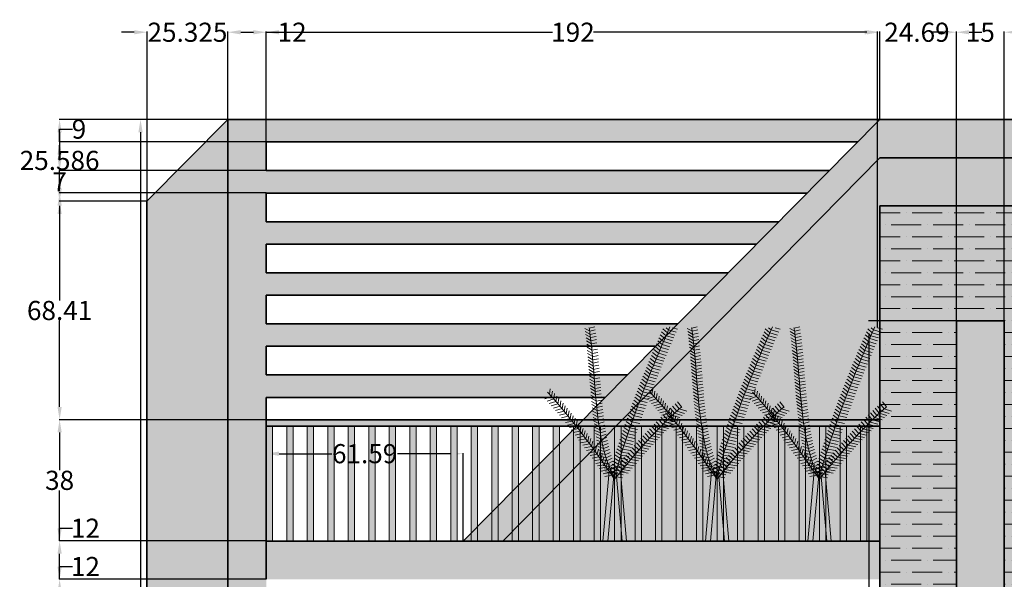
# Model space of a CAD drawing. Units: inches. Extents: x 184 to 649, y 215 to 818.
# Tile 8 of 9: x 184 to 492, y 643 to 818. Entities that reach past the tile are written whole.
import ezdxf

# ---------------------------------------------------------------- set-up
doc = ezdxf.new("R2010")
doc.units = ezdxf.units.IN
doc.header["$MEASUREMENT"] = 0
for name, color, linetype, lineweight in [('A-ANNO-DIMS', 2, 'Continuous', 18), ('A-ELEV', 7, 'Continuous', 35), ('A-ELEV-FILL', 9, 'Continuous', 13), ('A-ELEV-PATT', 8, 'Continuous', 13), ('A-ELEV-RAIL', 8, 'Continuous', 18), ('L-PLNT', 84, 'Continuous', 13)]:
    doc.layers.add(name, color=color, linetype=linetype, lineweight=lineweight)
doc.styles.get("Standard").update_dxf_attribs({"font": 'arial.ttf'})
doc.dimstyles.get("Standard").update_dxf_attribs({"dimtxt": 6, "dimasz": 4, "dimexe": 0.18, "dimexo": 0.0625, "dimgap": 0.09, "dimtad": 0, "dimtih": 1, "dimtoh": 1, "dimdec": 0, "dimzin": 0, "dimdsep": 46, "dimlunit": 3, "dimtxsty": 'Standard', "dimcen": 0.09, "dimadec": 0, "dimazin": 0, "dimtfac": 1, "dimtdec": 0, "dimtofl": 0, "dimtmove": 0, "dimatfit": 3, "dimfxl": 1, "dimtolj": 1, "dimtzin": 0, "dimarcsym": 0})

# ---------------------------------------------------------------- blocks, each defined once
blk = doc.blocks.new('PLANT-PALM')
for p, q in [((274.94, 416.06), (273.31, 416.97)), ((274.8, 417.06), (274.61, 417.16)), ((274.73, 417.05), (276.46, 417.47)), ((274.87, 416.06), (276.6, 416.47)), ((299.15, 415.59), (297.73, 416.77)), ((299.55, 416.5), (298.76, 417.16)), ((299.55, 416.5), (301.94, 415.78)), ((300.78, 417.16), (302.34, 416.68)), ((275.06, 415.07), (273.44, 415.99)), ((275.18, 414.08), (273.57, 415)), ((275.3, 413.08), (273.69, 414.02)), ((275.4, 412.09), (273.8, 413.03)), ((275, 415.07), (276.73, 415.46)), ((275.12, 414.07), (276.85, 414.46)), ((275.23, 413.08), (276.97, 413.45)), ((297.55, 411.92), (296.12, 413.09)), ((297.95, 412.84), (296.52, 414.01)), ((298.34, 413.75), (296.92, 414.93)), ((298.74, 414.67), (297.33, 415.85)), ((298.34, 413.75), (300.74, 413.04)), ((298.74, 414.67), (301.13, 413.96)), ((299.14, 415.59), (301.53, 414.87)), ((275.51, 411.09), (273.9, 412.04)), ((275.6, 410.1), (274, 411.05)), ((275.69, 409.1), (274.1, 410.06)), ((275.34, 412.09), (277.08, 412.45)), ((275.44, 411.09), (277.18, 411.45)), ((275.54, 410.1), (277.28, 410.45)), ((296.38, 409.16), (294.94, 410.32)), ((296.76, 410.08), (295.33, 411.24)), ((297.16, 411), (295.73, 412.16)), ((296.76, 410.08), (299.16, 409.39)), ((297.16, 411), (299.55, 410.3)), ((297.55, 411.92), (299.94, 411.22)), ((297.94, 412.84), (300.34, 412.13)), ((275.78, 408.11), (274.19, 409.06)), ((275.87, 407.11), (274.28, 408.07)), ((275.95, 406.11), (274.36, 407.08)), ((275.63, 409.1), (277.38, 409.45)), ((275.72, 408.1), (277.47, 408.45)), ((275.81, 407.11), (277.55, 407.44)), ((295.22, 406.39), (293.78, 407.54)), ((295.6, 407.31), (294.16, 408.46)), ((295.99, 408.23), (294.55, 409.39)), ((295.6, 407.31), (298.01, 406.64)), ((295.99, 408.24), (298.39, 407.56)), ((296.37, 409.16), (298.78, 408.47)), ((276.03, 405.12), (274.44, 406.08)), ((276.11, 404.12), (274.52, 405.08)), ((276.19, 403.12), (274.6, 404.09)), ((275.89, 406.11), (277.64, 406.45)), ((275.97, 405.11), (277.72, 405.45)), ((276.05, 404.12), (277.8, 404.45)), ((293.71, 402.68), (292.26, 403.82)), ((294.08, 403.61), (292.63, 404.75)), ((294.46, 404.54), (293.01, 405.68)), ((294.84, 405.46), (293.39, 406.61)), ((294.46, 404.54), (296.87, 403.88)), ((294.84, 405.46), (297.25, 404.8)), ((295.22, 406.39), (297.62, 405.72)), ((276.27, 402.13), (274.68, 403.09)), ((276.35, 401.13), (274.75, 402.09)), ((276.43, 400.13), (274.83, 401.09)), ((276.13, 403.12), (277.88, 403.45)), ((276.21, 402.12), (277.96, 402.46)), ((276.29, 401.13), (278.04, 401.46)), ((292.6, 399.9), (291.14, 401.02)), ((292.97, 400.83), (291.51, 401.95)), ((293.34, 401.76), (291.88, 402.89)), ((292.97, 400.83), (295.38, 400.2)), ((293.34, 401.76), (295.75, 401.12)), ((293.71, 402.68), (296.12, 402.04)), ((294.08, 403.61), (296.49, 402.96)), ((262.25, 396.34), (262.49, 398.02)), ((276.51, 399.14), (274.91, 400.09)), ((276.59, 398.14), (274.99, 399.09)), ((276.67, 397.14), (275.07, 398.09)), ((276.37, 400.13), (278.12, 400.47)), ((276.45, 399.13), (278.2, 399.47)), ((276.53, 398.14), (278.28, 398.48)), ((291.51, 397.1), (290.04, 398.21)), ((291.87, 398.03), (290.41, 399.15)), ((292.24, 398.97), (290.77, 400.08)), ((291.87, 398.03), (294.29, 397.42)), ((292.24, 398.97), (294.65, 398.35)), ((292.6, 399.9), (295.02, 399.27)), ((262.93, 395.59), (260.85, 394.94)), ((263.6, 394.85), (261.51, 394.21)), ((262.93, 395.6), (263.18, 397.28)), ((263.6, 394.85), (263.86, 396.53)), ((264.26, 394.11), (264.53, 395.78)), ((264.91, 393.35), (265.2, 395.02)), ((276.76, 396.15), (275.15, 397.08)), ((276.84, 395.15), (275.23, 396.08)), ((276.94, 394.16), (275.32, 395.08)), ((276.62, 397.14), (278.36, 397.49)), ((276.7, 396.14), (278.45, 396.5)), ((276.79, 395.15), (278.54, 395.51)), ((276.89, 394.15), (278.63, 394.52)), ((290.45, 394.3), (288.97, 395.4)), ((290.8, 395.23), (289.33, 396.34)), ((291.16, 396.17), (289.68, 397.27)), ((290.8, 395.23), (293.23, 394.64)), ((291.16, 396.17), (293.58, 395.57)), ((291.51, 397.1), (293.94, 396.5)), ((264.26, 394.1), (262.17, 393.48)), ((264.92, 393.35), (262.82, 392.74)), ((265.57, 392.59), (263.47, 391.99)), ((266.22, 391.82), (264.11, 391.25)), ((265.57, 392.59), (265.86, 394.26)), ((266.21, 391.83), (266.52, 393.5)), ((266.85, 391.06), (267.17, 392.73)), ((267.49, 390.29), (267.81, 391.95)), ((277.03, 393.16), (275.41, 394.07)), ((277.13, 392.17), (275.5, 393.07)), ((277.24, 391.17), (275.6, 392.06)), ((276.99, 393.16), (278.72, 393.54)), ((277.09, 392.16), (278.82, 392.55)), ((277.19, 391.17), (278.93, 391.57)), ((289.07, 390.54), (287.57, 391.62)), ((289.41, 391.48), (287.92, 392.57)), ((289.75, 392.42), (288.27, 393.51)), ((290.1, 393.36), (288.62, 394.45)), ((289.41, 391.48), (291.84, 390.92)), ((289.75, 392.42), (292.18, 391.85)), ((290.1, 393.36), (292.53, 392.78)), ((290.45, 394.3), (292.88, 393.71)), ((301.34, 390.38), (300.06, 391.94)), ((302.08, 391.06), (300.81, 392.62)), ((302.82, 391.73), (301.57, 393.3)), ((303.57, 392.39), (302.33, 393.98)), ((302.82, 391.73), (305.21, 391)), ((266.86, 391.06), (264.75, 390.49)), ((267.49, 390.29), (265.38, 389.73)), ((268.12, 389.51), (266.01, 388.97)), ((268.75, 388.73), (266.64, 388.2)), ((268.12, 389.51), (268.45, 391.17)), ((268.75, 388.73), (269.09, 390.39)), ((269.37, 387.95), (269.72, 389.61)), ((269.99, 387.16), (270.34, 388.82)), ((277.35, 390.18), (275.71, 391.05)), ((277.47, 389.19), (275.82, 390.05)), ((277.6, 388.2), (275.94, 389.04)), ((277.31, 390.18), (279.04, 390.59)), ((277.43, 389.18), (279.15, 389.61)), ((277.56, 388.19), (279.28, 388.63)), ((288.06, 387.72), (286.56, 388.79)), ((288.39, 388.66), (286.89, 389.73)), ((288.73, 389.6), (287.23, 390.68)), ((288.39, 388.66), (290.83, 388.12)), ((288.73, 389.6), (291.16, 389.05)), ((289.07, 390.54), (291.5, 389.98)), ((297.74, 386.91), (296.41, 388.42)), ((298.45, 387.62), (297.13, 389.14)), ((299.16, 388.32), (297.85, 389.85)), ((299.88, 389.01), (298.59, 390.55)), ((299.16, 388.32), (301.58, 387.68)), ((300.61, 389.7), (299.32, 391.25)), ((299.88, 389.01), (302.29, 388.36)), ((300.61, 389.7), (303.01, 389.03)), ((301.34, 390.38), (303.74, 389.69)), ((302.08, 391.06), (304.47, 390.35)), ((269.37, 387.95), (267.26, 387.43)), ((269.99, 387.16), (267.87, 386.65)), ((270.61, 386.37), (268.48, 385.87)), ((271.22, 385.58), (269.09, 385.09)), ((270.6, 386.37), (270.97, 388.03)), ((271.21, 385.58), (271.58, 387.24)), ((271.82, 384.79), (272.2, 386.44)), ((272.42, 383.99), (272.8, 385.64)), ((277.73, 387.21), (276.06, 388.03)), ((277.87, 386.22), (276.2, 387.03)), ((278.02, 385.23), (276.34, 386.02)), ((277.69, 387.2), (279.41, 387.66)), ((277.83, 386.21), (279.55, 386.69)), ((277.99, 385.22), (279.69, 385.72)), ((287.08, 384.88), (285.56, 385.94)), ((287.4, 385.83), (285.89, 386.89)), ((287.73, 386.77), (286.22, 387.84)), ((287.4, 385.83), (289.84, 385.31)), ((287.73, 386.77), (290.17, 386.25)), ((288.06, 387.72), (290.5, 387.18)), ((294.95, 384.05), (293.58, 385.53)), ((295.64, 384.77), (294.28, 386.26)), ((296.33, 385.49), (294.99, 386.98)), ((297.03, 386.2), (295.69, 387.71)), ((296.33, 385.49), (298.76, 384.92)), ((297.03, 386.2), (299.46, 385.61)), ((297.74, 386.91), (300.16, 386.31)), ((298.45, 387.62), (300.87, 387)), ((271.82, 384.79), (269.7, 384.3)), ((272.43, 383.99), (270.3, 383.51)), ((273.03, 383.19), (270.9, 382.72)), ((273.62, 382.39), (271.49, 381.93)), ((273.02, 383.19), (273.41, 384.84)), ((273.62, 382.39), (274.01, 384.04)), ((274.21, 381.58), (274.61, 383.23)), ((274.8, 380.78), (275.21, 382.42)), ((278.18, 384.24), (276.49, 385.01)), ((278.36, 383.26), (276.65, 384)), ((278.54, 382.28), (276.83, 382.99)), ((278.15, 384.24), (279.85, 384.75)), ((278.32, 383.25), (280.02, 383.79)), ((278.51, 382.27), (280.2, 382.83)), ((286.12, 382.04), (284.6, 383.08)), ((286.44, 382.99), (284.92, 384.03)), ((286.76, 383.94), (285.24, 384.98)), ((286.44, 382.99), (288.88, 382.49)), ((286.75, 383.94), (289.2, 383.43)), ((287.08, 384.88), (289.52, 384.37)), ((292.23, 381.11), (290.83, 382.56)), ((292.9, 381.85), (291.51, 383.31)), ((293.58, 382.59), (292.2, 384.05)), ((294.26, 383.32), (292.89, 384.79)), ((293.58, 382.59), (296.02, 382.07)), ((294.26, 383.32), (296.7, 382.79)), ((294.95, 384.05), (297.38, 383.5)), ((295.64, 384.77), (298.07, 384.21)), ((274.22, 381.58), (272.09, 381.13)), ((274.81, 380.78), (272.68, 380.33)), ((275.4, 379.97), (273.26, 379.53)), ((275.99, 379.16), (273.85, 378.72)), ((275.39, 379.97), (275.8, 381.61)), ((275.98, 379.16), (276.39, 380.8)), ((276.56, 378.35), (276.98, 379.99)), ((278.74, 381.3), (277.01, 381.99)), ((277.14, 377.53), (277.56, 379.18)), ((278.95, 380.32), (277.21, 380.98)), ((279.17, 379.35), (277.42, 379.97)), ((278.71, 381.29), (280.39, 381.87)), ((278.92, 380.31), (280.59, 380.92)), ((279.15, 379.34), (280.81, 379.98)), ((284.9, 378.23), (283.36, 379.24)), ((285.2, 379.18), (283.66, 380.2)), ((285.5, 380.14), (283.97, 381.16)), ((285.81, 381.09), (284.28, 382.12)), ((285.2, 379.18), (287.65, 378.72)), ((285.5, 380.14), (287.95, 379.67)), ((285.81, 381.09), (288.26, 380.61)), ((286.12, 382.04), (288.57, 381.55)), ((289.58, 378.12), (288.15, 379.54)), ((290.23, 378.87), (288.81, 380.3)), ((290.9, 379.63), (289.48, 381.06)), ((291.56, 380.37), (290.15, 381.81)), ((290.9, 379.63), (293.35, 379.16)), ((291.56, 380.37), (294.01, 379.89)), ((292.23, 381.11), (294.68, 380.62)), ((292.9, 381.85), (295.35, 381.35)), ((276.57, 378.35), (274.43, 377.92)), ((277.15, 377.53), (275.02, 377.11)), ((277.74, 376.72), (275.6, 376.3)), ((279.41, 378.38), (277.65, 378.97)), ((277.72, 376.72), (278.15, 378.36)), ((279.67, 377.41), (277.9, 377.96)), ((279.95, 376.45), (278.16, 376.96)), ((278.3, 375.9), (278.73, 377.55)), ((278.88, 375.09), (279.31, 376.73)), ((279.39, 378.37), (281.04, 379.04)), ((279.65, 377.4), (281.29, 378.11)), ((279.93, 376.44), (281.55, 377.18)), ((280.23, 375.49), (281.83, 376.27)), ((284.02, 375.36), (282.47, 376.36)), ((284.31, 376.32), (282.76, 377.32)), ((284.6, 377.27), (283.06, 378.28)), ((284.31, 376.32), (286.77, 375.89)), ((284.6, 377.28), (287.06, 376.83)), ((284.9, 378.23), (287.35, 377.78)), ((286.98, 375.08), (285.53, 376.47)), ((287.63, 375.84), (286.18, 377.24)), ((288.27, 376.61), (286.83, 378.01)), ((288.92, 377.36), (287.49, 378.78)), ((288.27, 376.61), (290.73, 376.18)), ((288.92, 377.36), (291.38, 376.93)), ((289.58, 378.12), (292.03, 377.67)), ((290.23, 378.87), (292.69, 378.42)), ((278.31, 375.91), (276.18, 375.49)), ((278.89, 375.09), (276.75, 374.67)), ((279.47, 374.27), (277.33, 373.86)), ((280.05, 373.46), (277.91, 373.04)), ((280.24, 375.49), (278.44, 375.96)), ((280.56, 374.55), (278.75, 374.97)), ((280.9, 373.61), (279.08, 373.97)), ((281.26, 372.67), (279.43, 372.98)), ((279.46, 374.27), (279.88, 375.91)), ((280.03, 373.45), (280.46, 375.09)), ((280.55, 374.54), (282.13, 375.36)), ((280.61, 372.64), (281.04, 374.28)), ((280.89, 373.6), (282.45, 374.46)), ((281.18, 371.82), (281.61, 373.46)), ((281.26, 372.67), (282.79, 373.58)), ((283.18, 372.48), (281.61, 373.46)), ((283.45, 373.44), (281.89, 374.43)), ((283.73, 374.4), (282.18, 375.39)), ((284.44, 371.99), (282.97, 373.36)), ((283.45, 373.44), (285.92, 373.04)), ((285.07, 372.76), (283.61, 374.14)), ((283.73, 374.4), (286.2, 373.99)), ((284.02, 375.36), (286.48, 374.94)), ((285.71, 373.54), (284.24, 374.92)), ((286.34, 374.31), (284.89, 375.7)), ((285.71, 373.54), (288.17, 373.15)), ((286.34, 374.31), (288.81, 373.91)), ((286.98, 375.08), (289.45, 374.67)), ((287.63, 375.84), (290.09, 375.43)), ((280.62, 372.64), (278.48, 372.23)), ((281.2, 371.82), (279.05, 371.41)), ((281.77, 371), (279.63, 370.59)), ((281.65, 371.75), (279.81, 372)), ((282.9, 371.52), (281.33, 372.49)), ((281.65, 371.75), (283.15, 372.7)), ((281.77, 371), (282.24, 372.12)), ((282.07, 370.84), (283.54, 371.85)), ((282.63, 370.56), (285.1, 370.19)), ((282.9, 371.52), (285.37, 371.14)), ((283.18, 372.48), (285.64, 372.09)), ((284.44, 371.99), (286.91, 371.62)), ((285.07, 372.76), (287.54, 372.39))]:
    blk.add_line(p, q)
blk.add_open_spline([(274.68, 417.16), (274.77, 416.57), (276.95, 400.47), (276.36, 381.5), (282.64, 369.73)], degree=3, knots=[87.299959, 87.299959, 87.299959, 87.299959, 88.780677, 127.704389, 127.704389, 127.704389, 127.704389])
for points in [[(282.63, 370.56), (286.61, 384.99), (292.84, 401.43), (299.95, 417.41)], [(282.55, 369.88), (275.93, 379.33), (269.31, 388.78), (261.65, 396.98)], [(282.64, 369.73), (290.67, 379.89), (297.61, 387.15), (303.65, 392.43)]]:
    blk.add_open_spline(points, degree=3)
blk = doc.blocks.new('PLANT-STEM')
for p, q in [((319.07, 530.29), (317.11, 508.48)), ((320.61, 530.15), (318.67, 508.48)), ((322.56, 530.1), (324.44, 508.48)), ((320.76, 528.67), (320.77, 508.48)), ((321.21, 529.98), (323.08, 508.48))]:
    blk.add_line(p, q)
blk = doc.blocks.new('*D10')
at = {"layer": 'A-ANNO-DIMS', "color": 0, "lineweight": -2, "transparency": 16777216}
for p, q in [((248.91, 786.73), (221.44, 786.73)), ((221.62, 782.73), (221.62, 519.88)), ((221.62, 250.73), (221.62, 513.57)), ((248.91, 246.73), (221.44, 246.73))]:
    blk.add_line(p, q, dxfattribs=at)
at = {"layer": 'A-ANNO-DIMS', "color": 0, "transparency": 16777216}
for points in [[(220.96, 782.73), (222.29, 782.73), (221.62, 786.73)], [(220.96, 250.73), (222.29, 250.73), (221.62, 246.73)]]:
    blk.add_solid(points, dxfattribs=at)
at = {"layer": 'Defpoints', "color": 0, "transparency": 16777216}
for p in [(221.62, 786.73), (248.97, 786.73), (248.97, 246.73)]:
    blk.add_point(p, dxfattribs=at)
at = {"layer": 'A-ANNO-DIMS', "color": 0, "transparency": 16777216, "insert": (221.62, 516.73), "char_height": 6, "attachment_point": 5}
blk.add_mtext('\\A1;540', dxfattribs=at)
blk = doc.blocks.new('*D19')
at = {"layer": 'A-ANNO-DIMS', "color": 0, "lineweight": -2, "transparency": 16777216}
for p, q in [((219.65, 814.08), (215.65, 814.08)), ((223.65, 761.2), (223.65, 814.26)), ((248.97, 786.79), (248.97, 814.26)), ((252.97, 814.08), (256.97, 814.08))]:
    blk.add_line(p, q, dxfattribs=at)
at = {"layer": 'A-ANNO-DIMS', "color": 0, "transparency": 16777216}
for points in [[(219.65, 814.74), (219.65, 813.41), (223.65, 814.08)], [(252.97, 814.74), (252.97, 813.41), (248.97, 814.08)]]:
    blk.add_solid(points, dxfattribs=at)
at = {"layer": 'Defpoints', "color": 0, "transparency": 16777216}
for p in [(248.97, 814.08), (248.97, 786.73), (223.65, 761.14)]:
    blk.add_point(p, dxfattribs=at)
at = {"layer": 'A-ANNO-DIMS', "color": 0, "transparency": 16777216, "insert": (236.31, 814.08), "char_height": 6, "attachment_point": 5}
blk.add_mtext('\\A1;25.325', dxfattribs=at)
blk = doc.blocks.new('*D20')
at = {"layer": 'A-ANNO-DIMS', "color": 0, "lineweight": -2, "transparency": 16777216}
for p, q in [((248.97, 786.79), (248.97, 814.26)), ((252.97, 814.08), (256.97, 814.08)), ((260.97, 779.79), (260.97, 814.26)), ((260.97, 814.08), (264.97, 814.08))]:
    blk.add_line(p, q, dxfattribs=at)
at = {"layer": 'A-ANNO-DIMS', "color": 0, "transparency": 16777216}
for points in [[(252.97, 814.74), (252.97, 813.41), (248.97, 814.08)], [(256.97, 814.74), (256.97, 813.41), (260.97, 814.08)]]:
    blk.add_solid(points, dxfattribs=at)
at = {"layer": 'Defpoints', "color": 0, "transparency": 16777216}
for p in [(260.97, 814.08), (248.97, 786.73), (260.97, 779.73)]:
    blk.add_point(p, dxfattribs=at)
at = {"layer": 'A-ANNO-DIMS', "color": 0, "transparency": 16777216, "insert": (269.05, 814.08), "char_height": 6, "attachment_point": 5}
blk.add_mtext('\\A1;12', dxfattribs=at)
blk = doc.blocks.new('*D21')
at = {"layer": 'A-ANNO-DIMS', "color": 0, "lineweight": -2, "transparency": 16777216}
for p, q in [((260.97, 779.79), (260.97, 814.26)), ((264.97, 814.08), (350.57, 814.08)), ((448.97, 814.08), (363.38, 814.08)), ((452.97, 786.79), (452.97, 814.26))]:
    blk.add_line(p, q, dxfattribs=at)
at = {"layer": 'A-ANNO-DIMS', "color": 0, "transparency": 16777216}
for points in [[(264.97, 814.74), (264.97, 813.41), (260.97, 814.08)], [(448.97, 814.74), (448.97, 813.41), (452.97, 814.08)]]:
    blk.add_solid(points, dxfattribs=at)
at = {"layer": 'Defpoints', "color": 0, "transparency": 16777216}
for p in [(452.97, 814.08), (452.97, 786.73), (260.97, 779.73)]:
    blk.add_point(p, dxfattribs=at)
at = {"layer": 'A-ANNO-DIMS', "color": 0, "transparency": 16777216, "insert": (356.97, 814.08), "char_height": 6, "attachment_point": 5}
blk.add_mtext('\\A1;192', dxfattribs=at)
blk = doc.blocks.new('*D22')
at = {"layer": 'A-ANNO-DIMS', "color": 0, "lineweight": -2, "transparency": 16777216}
for p, q in [((448.28, 814.08), (444.28, 814.08)), ((452.28, 721.59), (452.28, 814.26)), ((476.97, 723.79), (476.97, 814.26)), ((480.97, 814.08), (484.97, 814.08))]:
    blk.add_line(p, q, dxfattribs=at)
at = {"layer": 'A-ANNO-DIMS', "color": 0, "transparency": 16777216}
for points in [[(448.28, 814.74), (448.28, 813.41), (452.28, 814.08)], [(480.97, 814.74), (480.97, 813.41), (476.97, 814.08)]]:
    blk.add_solid(points, dxfattribs=at)
at = {"layer": 'Defpoints', "color": 0, "transparency": 16777216}
for p in [(476.97, 814.08), (452.28, 721.53), (476.97, 723.73)]:
    blk.add_point(p, dxfattribs=at)
at = {"layer": 'A-ANNO-DIMS', "color": 0, "transparency": 16777216, "insert": (464.63, 814.08), "char_height": 6, "attachment_point": 5}
blk.add_mtext('\\A1;24.69', dxfattribs=at)
blk = doc.blocks.new('*D23')
at = {"layer": 'A-ANNO-DIMS', "color": 0, "lineweight": -2, "transparency": 16777216}
for p, q in [((472.97, 814.08), (468.97, 814.08)), ((476.97, 723.79), (476.97, 814.26)), ((491.97, 723.79), (491.97, 814.26)), ((495.97, 814.08), (499.97, 814.08))]:
    blk.add_line(p, q, dxfattribs=at)
at = {"layer": 'A-ANNO-DIMS', "color": 0, "transparency": 16777216}
for points in [[(472.97, 814.74), (472.97, 813.41), (476.97, 814.08)], [(495.97, 814.74), (495.97, 813.41), (491.97, 814.08)]]:
    blk.add_solid(points, dxfattribs=at)
at = {"layer": 'Defpoints', "color": 0, "transparency": 16777216}
for p in [(491.97, 814.08), (476.97, 723.73), (491.97, 723.73)]:
    blk.add_point(p, dxfattribs=at)
at = {"layer": 'A-ANNO-DIMS', "color": 0, "transparency": 16777216, "insert": (484.47, 814.08), "char_height": 6, "attachment_point": 5}
blk.add_mtext('\\A1;15', dxfattribs=at)
blk = doc.blocks.new('*D39')
at = {"layer": 'A-ANNO-DIMS', "color": 0, "lineweight": -2, "transparency": 16777216}
for p, q in [((196.3, 642.73), (196.3, 646.73)), ((196.3, 646.73), (200.3, 646.73)), ((260.91, 642.73), (196.12, 642.73)), ((196.3, 634.73), (196.3, 638.73)), ((260.91, 630.73), (196.12, 630.73))]:
    blk.add_line(p, q, dxfattribs=at)
at = {"layer": 'A-ANNO-DIMS', "color": 0, "transparency": 16777216}
for points in [[(195.63, 638.73), (196.96, 638.73), (196.3, 642.73)], [(195.63, 634.73), (196.96, 634.73), (196.3, 630.73)]]:
    blk.add_solid(points, dxfattribs=at)
at = {"layer": 'Defpoints', "color": 0, "transparency": 16777216}
for p in [(196.3, 642.73), (260.97, 642.73), (260.97, 630.73)]:
    blk.add_point(p, dxfattribs=at)
at = {"layer": 'A-ANNO-DIMS', "color": 0, "transparency": 16777216, "insert": (204.37, 646.73), "char_height": 6, "attachment_point": 5}
blk.add_mtext('\\A1;12', dxfattribs=at)
blk = doc.blocks.new('*D40')
at = {"layer": 'A-ANNO-DIMS', "color": 0, "lineweight": -2, "transparency": 16777216}
for p, q in [((196.3, 654.73), (196.3, 658.73)), ((196.3, 658.73), (200.3, 658.73)), ((260.91, 654.73), (196.12, 654.73)), ((196.3, 646.73), (196.3, 650.73)), ((260.91, 642.73), (196.12, 642.73))]:
    blk.add_line(p, q, dxfattribs=at)
at = {"layer": 'A-ANNO-DIMS', "color": 0, "transparency": 16777216}
for points in [[(195.63, 650.73), (196.96, 650.73), (196.3, 654.73)], [(195.63, 646.73), (196.96, 646.73), (196.3, 642.73)]]:
    blk.add_solid(points, dxfattribs=at)
at = {"layer": 'Defpoints', "color": 0, "transparency": 16777216}
for p in [(196.3, 654.73), (260.97, 654.73), (260.97, 642.73)]:
    blk.add_point(p, dxfattribs=at)
at = {"layer": 'A-ANNO-DIMS', "color": 0, "transparency": 16777216, "insert": (204.37, 658.73), "char_height": 6, "attachment_point": 5}
blk.add_mtext('\\A1;12', dxfattribs=at)
blk = doc.blocks.new('*D41')
at = {"layer": 'A-ANNO-DIMS', "color": 0, "lineweight": -2, "transparency": 16777216}
for p, q in [((260.91, 692.73), (196.12, 692.73)), ((196.3, 688.73), (196.3, 676.88)), ((196.3, 658.73), (196.3, 670.57)), ((260.91, 654.73), (196.12, 654.73))]:
    blk.add_line(p, q, dxfattribs=at)
at = {"layer": 'A-ANNO-DIMS', "color": 0, "transparency": 16777216}
for points in [[(195.63, 688.73), (196.96, 688.73), (196.3, 692.73)], [(195.63, 658.73), (196.96, 658.73), (196.3, 654.73)]]:
    blk.add_solid(points, dxfattribs=at)
at = {"layer": 'Defpoints', "color": 0, "transparency": 16777216}
for p in [(196.3, 692.73), (260.97, 692.73), (260.97, 654.73)]:
    blk.add_point(p, dxfattribs=at)
at = {"layer": 'A-ANNO-DIMS', "color": 0, "transparency": 16777216, "insert": (196.3, 673.73), "char_height": 6, "attachment_point": 5}
blk.add_mtext('\\A1;38', dxfattribs=at)
blk = doc.blocks.new('*D42')
at = {"layer": 'A-ANNO-DIMS', "color": 0, "lineweight": -2, "transparency": 16777216}
for p, q in [((223.58, 761.14), (196.12, 761.14)), ((196.3, 757.14), (196.3, 730.09)), ((196.3, 696.73), (196.3, 723.78)), ((260.91, 692.73), (196.12, 692.73))]:
    blk.add_line(p, q, dxfattribs=at)
at = {"layer": 'A-ANNO-DIMS', "color": 0, "transparency": 16777216}
for points in [[(195.63, 757.14), (196.96, 757.14), (196.3, 761.14)], [(195.63, 696.73), (196.96, 696.73), (196.3, 692.73)]]:
    blk.add_solid(points, dxfattribs=at)
at = {"layer": 'Defpoints', "color": 0, "transparency": 16777216}
for p in [(196.3, 761.14), (223.65, 761.14), (260.97, 692.73)]:
    blk.add_point(p, dxfattribs=at)
at = {"layer": 'A-ANNO-DIMS', "color": 0, "transparency": 16777216, "insert": (196.3, 726.93), "char_height": 6, "attachment_point": 5}
blk.add_mtext('\\A1;68.41', dxfattribs=at)
blk = doc.blocks.new('*D43')
at = {"layer": 'A-ANNO-DIMS', "color": 0, "lineweight": -2, "transparency": 16777216}
for p, q in [((248.91, 786.73), (196.12, 786.73)), ((196.3, 782.73), (196.3, 777.09)), ((196.3, 765.14), (196.3, 770.78)), ((223.58, 761.14), (196.12, 761.14))]:
    blk.add_line(p, q, dxfattribs=at)
at = {"layer": 'A-ANNO-DIMS', "color": 0, "transparency": 16777216}
for points in [[(195.63, 782.73), (196.96, 782.73), (196.3, 786.73)], [(195.63, 765.14), (196.96, 765.14), (196.3, 761.14)]]:
    blk.add_solid(points, dxfattribs=at)
at = {"layer": 'Defpoints', "color": 0, "transparency": 16777216}
for p in [(196.3, 786.73), (248.97, 786.73), (223.65, 761.14)]:
    blk.add_point(p, dxfattribs=at)
at = {"layer": 'A-ANNO-DIMS', "color": 0, "transparency": 16777216, "insert": (196.3, 773.93), "char_height": 6, "attachment_point": 5}
blk.add_mtext('\\A1;25.586', dxfattribs=at)
blk = doc.blocks.new('*D54')
at = {"layer": 'A-ANNO-DIMS', "color": 0, "lineweight": -2, "transparency": 16777216}
for p, q in [((196.3, 779.73), (196.3, 783.73)), ((196.3, 783.73), (200.3, 783.73)), ((260.91, 779.73), (196.12, 779.73)), ((196.3, 774.73), (196.3, 775.73)), ((260.91, 770.73), (196.12, 770.73))]:
    blk.add_line(p, q, dxfattribs=at)
at = {"layer": 'A-ANNO-DIMS', "color": 0, "transparency": 16777216}
for points in [[(195.63, 775.73), (196.96, 775.73), (196.3, 779.73)], [(195.63, 774.73), (196.96, 774.73), (196.3, 770.73)]]:
    blk.add_solid(points, dxfattribs=at)
at = {"layer": 'Defpoints', "color": 0, "transparency": 16777216}
for p in [(196.3, 779.73), (260.97, 779.73), (260.97, 770.73)]:
    blk.add_point(p, dxfattribs=at)
at = {"layer": 'A-ANNO-DIMS', "color": 0, "transparency": 16777216, "insert": (202.36, 783.73), "char_height": 6, "attachment_point": 5}
blk.add_mtext('\\A1;9', dxfattribs=at)
blk = doc.blocks.new('*D55')
at = {"layer": 'A-ANNO-DIMS', "color": 0, "lineweight": -2, "transparency": 16777216}
for p, q in [((196.3, 774.73), (196.3, 778.73)), ((260.91, 770.73), (196.12, 770.73)), ((260.91, 763.73), (196.12, 763.73)), ((196.3, 759.73), (196.3, 755.73))]:
    blk.add_line(p, q, dxfattribs=at)
at = {"layer": 'A-ANNO-DIMS', "color": 0, "transparency": 16777216}
for points in [[(195.63, 774.73), (196.96, 774.73), (196.3, 770.73)], [(195.63, 759.73), (196.96, 759.73), (196.3, 763.73)]]:
    blk.add_solid(points, dxfattribs=at)
at = {"layer": 'Defpoints', "color": 0, "transparency": 16777216}
for p in [(196.3, 770.73), (260.97, 770.73), (260.97, 763.73)]:
    blk.add_point(p, dxfattribs=at)
at = {"layer": 'A-ANNO-DIMS', "color": 0, "transparency": 16777216, "insert": (196.3, 767.23), "char_height": 6, "attachment_point": 5}
blk.add_mtext('\\A1;7', dxfattribs=at)
blk = doc.blocks.new('*D56')
at = {"layer": 'A-ANNO-DIMS', "color": 0, "lineweight": -2, "transparency": 16777216}
for p, q in [((260.97, 654.79), (260.97, 682.26)), ((264.97, 682.08), (281.53, 682.08)), ((318.57, 682.08), (302.01, 682.08)), ((322.57, 654.79), (322.57, 682.26))]:
    blk.add_line(p, q, dxfattribs=at)
at = {"layer": 'A-ANNO-DIMS', "color": 0, "transparency": 16777216}
for points in [[(264.97, 682.74), (264.97, 681.41), (260.97, 682.08)], [(318.57, 682.74), (318.57, 681.41), (322.57, 682.08)]]:
    blk.add_solid(points, dxfattribs=at)
at = {"layer": 'Defpoints', "color": 0, "transparency": 16777216}
for p in [(322.57, 682.08), (260.97, 654.73), (322.57, 654.73)]:
    blk.add_point(p, dxfattribs=at)
at = {"layer": 'A-ANNO-DIMS', "color": 0, "transparency": 16777216, "insert": (291.77, 682.08), "char_height": 6, "attachment_point": 5}
blk.add_mtext('\\A1;61.59', dxfattribs=at)
blk = doc.blocks.new('*D63')
at = {"layer": 'A-ANNO-DIMS', "color": 0, "lineweight": -2, "transparency": 16777216}
for p, q in [((476.91, 723.73), (449.44, 723.73)), ((449.62, 719.73), (449.62, 603.63)), ((449.62, 481.22), (449.62, 597.32)), ((476.91, 477.22), (449.44, 477.22))]:
    blk.add_line(p, q, dxfattribs=at)
at = {"layer": 'A-ANNO-DIMS', "color": 0, "transparency": 16777216}
for points in [[(448.96, 719.73), (450.29, 719.73), (449.62, 723.73)], [(448.96, 481.22), (450.29, 481.22), (449.62, 477.22)]]:
    blk.add_solid(points, dxfattribs=at)
at = {"layer": 'Defpoints', "color": 0, "transparency": 16777216}
for p in [(449.62, 723.73), (476.97, 723.73), (476.97, 477.22)]:
    blk.add_point(p, dxfattribs=at)
at = {"layer": 'A-ANNO-DIMS', "color": 0, "transparency": 16777216, "insert": (449.62, 600.47), "char_height": 6, "attachment_point": 5}
blk.add_mtext('\\A1;246.5', dxfattribs=at)

msp = doc.modelspace()

# ---------------------------------------------------------------- hatches: boundary and pattern name
at = {"layer": 'A-ELEV-FILL'}
h = msp.add_hatch(color=256, dxfattribs=at)
h.dxf.hatch_style = 1
h.paths.add_polyline_path([(248.9726, 786.7265), (223.6471, 761.141), (223.6471, 257.141), (248.9726, 246.7265)])
h = msp.add_hatch(color=256, dxfattribs=at)
h.dxf.hatch_style = 1
h.paths.add_polyline_path([(452.9726, 369.7265), (248.9726, 369.7265), (248.9726, 246.7265), (275.9726, 246.7265), (275.9726, 328.7265), (437.9726, 328.7265), (437.9726, 246.7265), (446.6666, 246.7265), (452.9726, 282.7265)])
h.paths.add_polyline_path([(275.9726, 340.7265), (275.9726, 354.7265), (437.9726, 354.7265), (437.9726, 340.7265)], flags=16)
h.paths.add_polyline_path([(452.9726, 510.7265), (260.9726, 510.7265), (260.9726, 642.7265), (260.9726, 699.7265), (367.0226, 699.7265), (373.9381, 706.7265), (260.9726, 706.7265), (260.9726, 715.7265), (382.8295, 715.7265), (389.745, 722.7265), (260.9726, 722.7265), (260.9726, 731.7265), (398.6364, 731.7265), (405.5519, 738.7265), (260.9726, 738.7265), (260.9726, 747.7265), (414.4433, 747.7265), (421.3588, 754.7265), (260.9726, 754.7265), (260.9726, 763.7265), (430.2502, 763.7265), (437.1657, 770.7265), (260.9726, 770.7265), (260.9726, 779.7265), (446.057, 779.7265), (452.9726, 786.7265), (248.9726, 786.7265), (248.9726, 369.7265), (260.9726, 369.7265), (260.9726, 498.7265), (452.9726, 498.7265)])
h = msp.add_hatch(color=256, dxfattribs=at)
h.dxf.hatch_style = 1
h.paths.add_polyline_path([(608.9726, 786.7265), (452.9726, 786.7265), (360.1071, 692.7265), (372.3627, 692.7265), (452.9726, 774.7265), (596.9726, 774.7265), (596.9726, 369.7265), (581.9726, 369.7265), (581.9726, 282.7265), (594.8393, 246.7265), (608.9726, 246.7265)])
h = msp.add_hatch(color=256, dxfattribs=at)
h.dxf.hatch_style = 1
h.paths.add_polyline_path([(596.9726, 774.7265), (452.9726, 774.7265), (372.3627, 692.7265), (386.4196, 692.7265), (452.9726, 759.7265), (581.9726, 759.7265)])
h = msp.add_hatch(color=256, dxfattribs=at)
h.dxf.hatch_style = 1
h.paths.add_polyline_path([(452.9726, 759.7265), (386.4196, 692.7265), (452.9726, 692.7265)])
h = msp.add_hatch(color=256, dxfattribs=at)
h.dxf.hatch_style = 1
h.paths.add_polyline_path([(521.9726, 759.7265), (452.9726, 759.7265), (452.9726, 441.2233), (521.9726, 441.2233)])
h.paths.add_polyline_path([(491.9726, 477.2233), (476.9726, 477.2233), (476.9726, 723.7265), (491.9726, 723.7265)], flags=16)
h = msp.add_hatch(color=256, dxfattribs=at)
h.dxf.hatch_style = 1
h.paths.add_polyline_path([(491.9726, 723.7265), (476.9726, 723.7265), (476.9726, 477.2233), (491.9726, 477.2233)])
h = msp.add_hatch(color=256, dxfattribs=at)
h.dxf.hatch_style = 1
h.paths.add_polyline_path([(360.1071, 692.7265), (260.9726, 692.7265), (260.9726, 690.7265), (358.1312, 690.7265)])
h.paths.add_polyline_path([(262.9726, 690.7265), (260.9726, 690.7265), (260.9726, 654.7265), (262.9726, 654.7265)])
h.paths.add_polyline_path([(269.3864, 690.7265), (267.3864, 690.7265), (267.3864, 654.7265), (269.3864, 654.7265)])
h.paths.add_polyline_path([(275.8001, 690.7265), (273.8001, 690.7265), (273.8001, 654.7265), (275.8001, 654.7265)])
h.paths.add_polyline_path([(282.2139, 690.7265), (280.2139, 690.7265), (280.2139, 654.7265), (282.2139, 654.7265)])
h.paths.add_polyline_path([(288.6277, 690.7265), (286.6277, 690.7265), (286.6277, 654.7265), (288.6277, 654.7265)])
h.paths.add_polyline_path([(295.0415, 690.7265), (293.0415, 690.7265), (293.0415, 654.7265), (295.0415, 654.7265)])
h.paths.add_polyline_path([(301.4553, 690.7265), (299.4553, 690.7265), (299.4553, 654.7265), (301.4553, 654.7265)])
h.paths.add_polyline_path([(307.8691, 690.7265), (305.8691, 690.7265), (305.8691, 654.7265), (307.8691, 654.7265)])
h.paths.add_polyline_path([(314.2829, 690.7265), (312.2829, 690.7265), (312.2829, 654.7265), (314.2829, 654.7265)])
h.paths.add_polyline_path([(320.6967, 690.7265), (318.6967, 690.7265), (318.6967, 654.7265), (320.6967, 654.7265)])
h.paths.add_polyline_path([(327.1105, 690.7265), (325.1105, 690.7265), (325.1105, 657.3024), (327.1105, 659.3269)])
h.paths.add_polyline_path([(333.5243, 690.7265), (331.5243, 690.7265), (331.5243, 663.7946), (333.5243, 665.819)])
h.paths.add_polyline_path([(339.9381, 690.7265), (337.9381, 690.7265), (337.9381, 670.2867), (339.9381, 672.3112)])
h.paths.add_polyline_path([(346.3519, 690.7265), (344.3519, 690.7265), (344.3519, 676.7789), (346.3519, 678.8033)])
h.paths.add_polyline_path([(352.7657, 690.7265), (350.7657, 690.7265), (350.7657, 683.271), (352.7657, 685.2955)])
h.paths.add_polyline_path([(358.1312, 690.7265), (357.1795, 690.7265), (357.1795, 689.7632)], flags=17)
h.paths.add_polyline_path([(372.3627, 692.7265), (360.1071, 692.7265), (358.1312, 690.7265), (370.3966, 690.7265)])
h.paths.add_polyline_path([(452.9726, 692.7265), (372.3627, 692.7265), (370.3966, 690.7265), (452.9726, 690.7265)])
h.paths.add_polyline_path([(448.9726, 690.7265), (446.9726, 690.7265), (446.9726, 654.7265), (448.9726, 654.7265)])
h.paths.add_polyline_path([(442.5588, 690.7265), (440.5588, 690.7265), (440.5588, 654.7265), (442.5588, 654.7265)])
h.paths.add_polyline_path([(436.145, 690.7265), (434.145, 690.7265), (434.145, 654.7265), (436.145, 654.7265)])
h.paths.add_polyline_path([(429.7312, 690.7265), (427.7312, 690.7265), (427.7312, 654.7265), (429.7312, 654.7265)])
h.paths.add_polyline_path([(423.3174, 690.7265), (421.3174, 690.7265), (421.3174, 654.7265), (423.3174, 654.7265)])
h.paths.add_polyline_path([(416.9036, 690.7265), (414.9036, 690.7265), (414.9036, 654.7265), (416.9036, 654.7265)])
h.paths.add_polyline_path([(410.4898, 690.7265), (408.4898, 690.7265), (408.4898, 654.7265), (410.4898, 654.7265)])
h.paths.add_polyline_path([(404.076, 690.7265), (402.076, 690.7265), (402.076, 654.7265), (404.076, 654.7265)])
h.paths.add_polyline_path([(397.6622, 690.7265), (395.6622, 690.7265), (395.6622, 654.7265), (397.6622, 654.7265)])
h.paths.add_polyline_path([(391.2484, 690.7265), (389.2484, 690.7265), (389.2484, 654.7265), (391.2484, 654.7265)])
h.paths.add_polyline_path([(384.8346, 690.7265), (382.8346, 690.7265), (382.8346, 654.7265), (384.8346, 654.7265)])
h.paths.add_polyline_path([(378.4208, 690.7265), (376.4208, 690.7265), (376.4208, 654.7265), (378.4208, 654.7265)])
h.paths.add_polyline_path([(372.007, 690.7265), (370.3966, 690.7265), (370.007, 690.3302), (370.007, 654.7265), (372.007, 654.7265)])
h.paths.add_polyline_path([(365.5932, 685.8403), (363.5932, 683.8058), (363.5932, 654.7265), (365.5932, 654.7265)])
h.paths.add_polyline_path([(359.1795, 679.3159), (357.1795, 677.2814), (357.1795, 654.7265), (359.1795, 654.7265)])
h.paths.add_polyline_path([(352.7657, 672.7915), (350.7657, 670.757), (350.7657, 654.7265), (352.7657, 654.7265)])
h.paths.add_polyline_path([(346.3519, 666.2671), (344.3519, 664.2326), (344.3519, 654.7265), (346.3519, 654.7265)])
h.paths.add_polyline_path([(339.9381, 659.7427), (337.9381, 657.7082), (337.9381, 654.7265), (339.9381, 654.7265)])
h.paths.add_polyline_path([(327.1105, 659.3269), (325.1105, 657.3024), (325.1105, 654.7265), (327.1105, 654.7265)])
h.paths.add_polyline_path([(333.5243, 665.819), (331.5243, 663.7946), (331.5243, 654.7265), (333.5243, 654.7265)])
h.paths.add_polyline_path([(339.9381, 672.3112), (337.9381, 670.2867), (337.9381, 657.7082), (339.9381, 659.7427)])
h.paths.add_polyline_path([(346.3519, 678.8033), (344.3519, 676.7789), (344.3519, 664.2326), (346.3519, 666.2671)])
h.paths.add_polyline_path([(352.7657, 685.2955), (350.7657, 683.271), (350.7657, 670.757), (352.7657, 672.7915)])
h.paths.add_polyline_path([(359.1795, 690.7265), (358.1312, 690.7265), (357.1795, 689.7632), (357.1795, 677.2814), (359.1795, 679.3159)])
h.paths.add_polyline_path([(365.5932, 690.7265), (363.5932, 690.7265), (363.5932, 683.8058), (365.5932, 685.8403)])
h.paths.add_polyline_path([(370.3966, 690.7265), (370.007, 690.7265), (370.007, 690.3302)], flags=17)
h = msp.add_hatch(color=256, dxfattribs=at)
h.dxf.hatch_style = 1
h.paths.add_polyline_path([(370.007, 690.3302), (370.007, 690.7265), (365.5932, 690.7265), (365.5932, 685.8403)])
h.paths.add_polyline_path([(363.5932, 690.7265), (359.1795, 690.7265), (359.1795, 679.3159), (363.5932, 683.8058)])
h.paths.add_polyline_path([(357.1795, 689.7632), (352.7657, 685.2955), (352.7657, 672.7915), (357.1795, 677.2814)])
h.paths.add_polyline_path([(350.7657, 683.271), (346.3519, 678.8033), (346.3519, 666.2671), (350.7657, 670.757)])
h.paths.add_polyline_path([(344.3519, 676.7789), (339.9381, 672.3112), (339.9381, 659.7427), (344.3519, 664.2326)])
h.paths.add_polyline_path([(337.9381, 670.2867), (333.5243, 665.819), (333.5243, 654.7265), (335.007, 654.7265), (337.9381, 657.7082)])
h.paths.add_polyline_path([(331.5243, 663.7946), (327.1105, 659.3269), (327.1105, 654.7265), (331.5243, 654.7265)])
h.paths.add_polyline_path([(325.1105, 657.3024), (322.5657, 654.7265), (325.1105, 654.7265)])
h = msp.add_hatch(color=256, dxfattribs=at)
h.dxf.hatch_style = 1
h.paths.add_polyline_path([(452.9726, 690.7265), (448.9726, 690.7265), (448.9726, 654.7265), (452.9726, 654.7265)])
h.paths.add_polyline_path([(446.9726, 690.7265), (442.5588, 690.7265), (442.5588, 654.7265), (446.9726, 654.7265)])
h.paths.add_polyline_path([(440.5588, 690.7265), (436.145, 690.7265), (436.145, 654.7265), (440.5588, 654.7265)])
h.paths.add_polyline_path([(434.145, 690.7265), (429.7312, 690.7265), (429.7312, 654.7265), (434.145, 654.7265)])
h.paths.add_polyline_path([(427.7312, 690.7265), (423.3174, 690.7265), (423.3174, 654.7265), (427.7312, 654.7265)])
h.paths.add_polyline_path([(421.3174, 690.7265), (416.9036, 690.7265), (416.9036, 654.7265), (421.3174, 654.7265)])
h.paths.add_polyline_path([(414.9036, 690.7265), (410.4898, 690.7265), (410.4898, 654.7265), (414.9036, 654.7265)])
h.paths.add_polyline_path([(408.4898, 690.7265), (404.076, 690.7265), (404.076, 654.7265), (408.4898, 654.7265)])
h.paths.add_polyline_path([(402.076, 690.7265), (397.6622, 690.7265), (397.6622, 654.7265), (402.076, 654.7265)])
h.paths.add_polyline_path([(395.6622, 690.7265), (391.2484, 690.7265), (391.2484, 654.7265), (395.6622, 654.7265)])
h.paths.add_polyline_path([(389.2484, 690.7265), (384.8346, 690.7265), (384.8346, 654.7265), (389.2484, 654.7265)])
h.paths.add_polyline_path([(382.8346, 690.7265), (378.4208, 690.7265), (378.4208, 654.7265), (382.8346, 654.7265)])
h.paths.add_polyline_path([(376.4208, 690.7265), (372.007, 690.7265), (372.007, 654.7265), (376.4208, 654.7265)])
h.paths.add_polyline_path([(370.007, 690.3302), (365.5932, 685.8403), (365.5932, 654.7265), (370.007, 654.7265)])
h.paths.add_polyline_path([(357.1795, 677.2814), (352.7657, 672.7915), (352.7657, 654.7265), (357.1795, 654.7265)])
h.paths.add_polyline_path([(363.5932, 683.8058), (359.1795, 679.3159), (359.1795, 654.7265), (363.5932, 654.7265)])
h.paths.add_polyline_path([(350.7657, 670.757), (346.3519, 666.2671), (346.3519, 654.7265), (350.7657, 654.7265)])
h.paths.add_polyline_path([(344.3519, 664.2326), (339.9381, 659.7427), (339.9381, 654.7265), (344.3519, 654.7265)])
h.paths.add_polyline_path([(337.9381, 657.7082), (335.007, 654.7265), (337.9381, 654.7265)])
h = msp.add_hatch(color=256, dxfattribs=at)
h.dxf.hatch_style = 1
h.paths.add_polyline_path([(452.9726, 654.7265), (260.9726, 654.7265), (260.9726, 642.7265), (452.9726, 642.7265)])
at = {"layer": 'A-ELEV-PATT'}
h = msp.add_hatch(dxfattribs=at)
h.set_pattern_fill('ANSI36', color=256, scale=30, angle=135)
h.paths.add_polyline_path([(521.9726, 759.7265), (452.9726, 759.7265), (452.9726, 441.2233), (521.9726, 441.2233)])
h.paths.add_polyline_path([(476.9726, 723.7265), (491.9726, 723.7265), (491.9726, 477.2233), (476.9726, 477.2233)], flags=16)

# ---------------------------------------------------------------- linework, layer by layer
at = {"layer": 'A-ELEV'}
for p, q in [((248.9726, 786.7265), (223.6471, 761.141)), ((608.9726, 786.7265), (248.9726, 786.7265)), ((248.9726, 786.7265), (248.9726, 246.7265)), ((452.9726, 786.7265), (322.5657, 654.7265)), ((260.9726, 779.7265), (260.9726, 770.7265)), ((446.057, 779.7265), (260.9726, 779.7265)), ((452.9726, 774.7265), (335.007, 654.7265)), ((596.9726, 774.7265), (452.9726, 774.7265)), ((437.1657, 770.7265), (260.9726, 770.7265)), ((260.9726, 763.7265), (260.9726, 754.7265)), ((430.2502, 763.7265), (260.9726, 763.7265)), ((223.6471, 761.141), (223.6471, 257.141)), ((581.9726, 759.7265), (452.9726, 759.7265)), ((452.9726, 441.2233), (452.9726, 759.7265)), ((421.3588, 754.7265), (260.9726, 754.7265)), ((260.9726, 747.7265), (260.9726, 738.7265)), ((414.4433, 747.7265), (260.9726, 747.7265)), ((405.5519, 738.7265), (260.9726, 738.7265)), ((260.9726, 731.7265), (260.9726, 722.7265)), ((398.6364, 731.7265), (260.9726, 731.7265)), ((389.745, 722.7265), (260.9726, 722.7265)), ((476.9726, 723.7265), (491.9726, 723.7265)), ((476.9726, 477.2233), (476.9726, 723.7265)), ((491.9726, 477.2233), (491.9726, 723.7265)), ((260.9726, 715.7265), (260.9726, 706.7265)), ((382.8295, 715.7265), (260.9726, 715.7265)), ((373.9381, 706.7265), (260.9726, 706.7265)), ((260.9726, 699.7265), (260.9726, 642.7265)), ((367.0226, 699.7265), (260.9726, 699.7265)), ((452.9726, 692.7265), (260.9726, 692.7265)), ((452.9726, 690.7265), (260.9726, 690.7265)), ((452.9726, 654.7265), (260.9726, 654.7265))]:
    msp.add_line(p, q, dxfattribs=at)
at = {"layer": 'A-ELEV-RAIL'}
for p, q in [((262.9726, 654.7265), (262.9726, 690.7265)), ((267.3864, 654.7265), (267.3864, 690.7265)), ((269.3864, 654.7265), (269.3864, 690.7265)), ((273.8001, 654.7265), (273.8001, 690.7265)), ((275.8001, 654.7265), (275.8001, 690.7265)), ((280.2139, 654.7265), (280.2139, 690.7265)), ((282.2139, 654.7265), (282.2139, 690.7265)), ((286.6277, 654.7265), (286.6277, 690.7265)), ((288.6277, 654.7265), (288.6277, 690.7265)), ((293.0415, 654.7265), (293.0415, 690.7265)), ((295.0415, 654.7265), (295.0415, 690.7265)), ((299.4553, 654.7265), (299.4553, 690.7265)), ((301.4553, 654.7265), (301.4553, 690.7265)), ((305.8691, 654.7265), (305.8691, 690.7265)), ((307.8691, 654.7265), (307.8691, 690.7265)), ((312.2829, 654.7265), (312.2829, 690.7265)), ((314.2829, 654.7265), (314.2829, 690.7265)), ((318.6967, 654.7265), (318.6967, 690.7265)), ((320.6967, 654.7265), (320.6967, 690.7265)), ((325.1105, 654.7265), (325.1105, 690.7265)), ((327.1105, 654.7265), (327.1105, 690.7265)), ((331.5243, 654.7265), (331.5243, 690.7265)), ((333.5243, 654.7265), (333.5243, 690.7265)), ((337.9381, 654.7265), (337.9381, 690.7265)), ((339.9381, 654.7265), (339.9381, 690.7265)), ((344.3519, 654.7265), (344.3519, 690.7265)), ((346.3519, 654.7265), (346.3519, 690.7265)), ((350.7657, 654.7265), (350.7657, 690.7265)), ((352.7657, 654.7265), (352.7657, 690.7265)), ((357.1795, 654.7265), (357.1795, 690.7265)), ((359.1795, 654.7265), (359.1795, 690.7265)), ((363.5932, 654.7265), (363.5932, 690.7265)), ((365.5932, 654.7265), (365.5932, 690.7265)), ((370.007, 654.7265), (370.007, 690.7265)), ((372.007, 654.7265), (372.007, 690.7265)), ((376.4208, 654.7265), (376.4208, 690.7265)), ((378.4208, 654.7265), (378.4208, 690.7265)), ((382.8346, 654.7265), (382.8346, 690.7265)), ((384.8346, 654.7265), (384.8346, 690.7265)), ((389.2484, 654.7265), (389.2484, 690.7265)), ((391.2484, 654.7265), (391.2484, 690.7265)), ((395.6622, 654.7265), (395.6622, 690.7265)), ((397.6622, 654.7265), (397.6622, 690.7265)), ((402.076, 654.7265), (402.076, 690.7265)), ((404.076, 654.7265), (404.076, 690.7265)), ((408.4898, 654.7265), (408.4898, 690.7265)), ((410.4898, 654.7265), (410.4898, 690.7265)), ((414.9036, 654.7265), (414.9036, 690.7265)), ((416.9036, 654.7265), (416.9036, 690.7265)), ((421.3174, 654.7265), (421.3174, 690.7265)), ((423.3174, 654.7265), (423.3174, 690.7265)), ((427.7312, 654.7265), (427.7312, 690.7265)), ((429.7312, 654.7265), (429.7312, 690.7265)), ((434.145, 654.7265), (434.145, 690.7265)), ((436.145, 654.7265), (436.145, 690.7265)), ((440.5588, 654.7265), (440.5588, 690.7265)), ((442.5588, 654.7265), (442.5588, 690.7265)), ((446.9726, 654.7265), (446.9726, 690.7265)), ((448.9726, 654.7265), (448.9726, 690.7265))]:
    msp.add_line(p, q, dxfattribs=at)

# ---------------------------------------------------------------- block references
at = {"layer": 'L-PLNT'}
for name, p in [('PLANT-PALM', (87.3613, 304.3643)), ('PLANT-PALM', (119.4303, 304.3643)), ('PLANT-PALM', (151.4993, 304.3643)), ('PLANT-STEM', (49.2394, 146.249)), ('PLANT-STEM', (81.3084, 146.249)), ('PLANT-STEM', (113.3773, 146.249))]:
    msp.add_blockref(name, p, dxfattribs=at)

# ---------------------------------------------------------------- dimensions: what is measured, and where the dimension line sits
at = {"layer": 'A-ANNO-DIMS'}
for base, p1, p2, override, picture, middle in [((248.97256, 814.07655), (223.64709, 761.14099), (248.97256, 786.72655), {"dimdec": 3, "dimlfac": 1, "dimrnd": 0, "dimzin": 0, "dimdsep": 46, "dimlunit": 2}, '*D19', (236.30982, 814.07655)), ((260.9726, 814.0765), (248.9726, 786.7265), (260.9726, 779.7265), {"dimdec": 0, "dimlfac": 1, "dimrnd": 0, "dimzin": 0, "dimdsep": 46, "dimlunit": 2}, '*D20', (269.0469, 814.0765)), ((452.9726, 814.0765), (260.9726, 779.7265), (452.9726, 786.7265), {"dimdec": 0, "dimlfac": 1, "dimrnd": 0, "dimzin": 0, "dimdsep": 46, "dimlunit": 2}, '*D21', (356.9726, 814.0765)), ((476.9726, 814.0765), (452.2819, 721.525), (476.9726, 723.7265), {"dimdec": 2, "dimlfac": 1, "dimrnd": 0, "dimzin": 0, "dimdsep": 46, "dimlunit": 2}, '*D22', (464.6272, 814.0765)), ((491.9726, 814.0765), (476.9726, 723.7265), (491.9726, 723.7265), {"dimdec": 0, "dimlfac": 1, "dimrnd": 0, "dimzin": 0, "dimdsep": 46, "dimlunit": 2}, '*D23', (484.4726, 814.0765)), ((322.5657, 682.0765), (260.9726, 654.7265), (322.5657, 654.7265), {"dimdec": 2, "dimlfac": 1, "dimrnd": 0, "dimzin": 0, "dimdsep": 46, "dimlunit": 2}, '*D56', (291.7691, 682.0765))]:
    dim = msp.add_linear_dim(base=base, p1=p1, p2=p2, dimstyle='Standard', override=override, dxfattribs=at)
    dim.commit()
    dim.dimension.update_dxf_attribs({"geometry": picture, "text_midpoint": middle})
for base, p1, p2, override, picture, middle in [((196.29709, 786.72655), (223.64709, 761.14099), (248.97256, 786.72655), {"dimdec": 3, "dimlfac": 1, "dimrnd": 0, "dimzin": 0, "dimdsep": 46, "dimlunit": 2}, '*D43', (196.29709, 773.93377)), ((196.2971, 779.7265), (260.9726, 770.7265), (260.9726, 779.7265), {"dimdec": 0, "dimlfac": 1, "dimrnd": 0, "dimzin": 0, "dimdsep": 46, "dimlunit": 2}, '*D54', (202.3598, 783.7265)), ((221.6226, 786.7265), (248.9726, 246.7265), (248.9726, 786.7265), {"dimdec": 0, "dimlfac": 1, "dimrnd": 0, "dimzin": 0, "dimdsep": 46, "dimlunit": 2}, '*D10', (221.6226, 516.7265)), ((196.2971, 770.7265), (260.9726, 763.7265), (260.9726, 770.7265), {"dimdec": 0, "dimlfac": 1, "dimrnd": 0, "dimzin": 0, "dimdsep": 46, "dimlunit": 2}, '*D55', (196.2971, 767.2265)), ((196.2971, 761.141), (260.9726, 692.7265), (223.6471, 761.141), {"dimdec": 2, "dimlfac": 1, "dimrnd": 0, "dimzin": 0, "dimdsep": 46, "dimlunit": 2}, '*D42', (196.2971, 726.9338)), ((449.6226, 723.7265), (476.9726, 477.2233), (476.9726, 723.7265), {"dimdec": 1, "dimlfac": 1, "dimrnd": 0, "dimzin": 0, "dimdsep": 46, "dimlunit": 2}, '*D63', (449.6226, 600.4749)), ((196.2971, 692.7265), (260.9726, 654.7265), (260.9726, 692.7265), {"dimdec": 0, "dimlfac": 1, "dimrnd": 0, "dimzin": 0, "dimdsep": 46, "dimlunit": 2}, '*D41', (196.2971, 673.7265)), ((196.2971, 654.7265), (260.9726, 642.7265), (260.9726, 654.7265), {"dimdec": 0, "dimlfac": 1, "dimrnd": 0, "dimzin": 0, "dimdsep": 46, "dimlunit": 2}, '*D40', (204.3714, 658.7265)), ((196.2971, 642.7265), (260.9726, 630.7265), (260.9726, 642.7265), {"dimdec": 0, "dimlfac": 1, "dimrnd": 0, "dimzin": 0, "dimdsep": 46, "dimlunit": 2}, '*D39', (204.3714, 646.7265))]:
    dim = msp.add_linear_dim(base=base, p1=p1, p2=p2, angle=90, dimstyle='Standard', override=override, dxfattribs=at)
    dim.commit()
    dim.dimension.update_dxf_attribs({"geometry": picture, "text_midpoint": middle})

doc.saveas('drawing.dxf')
